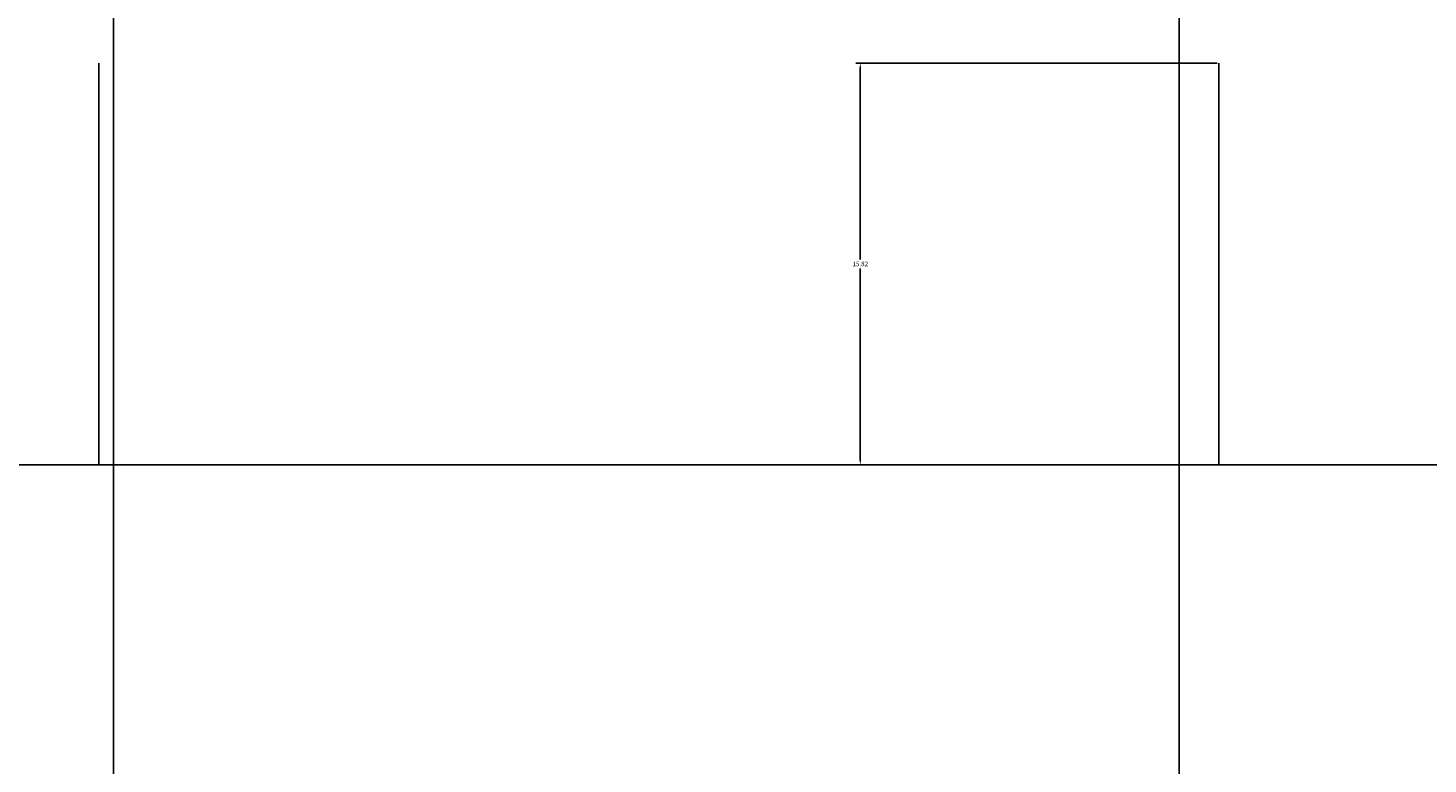
# Model space of a CAD drawing. Units: millimetres. Extents: x -8 to 285, y 5 to 221.
# Tile 21 of 30: x 186 to 241, y 103 to 132. Entities that reach past the tile are written whole.
import ezdxf

# ---------------------------------------------------------------- set-up
doc = ezdxf.new("R2010")
doc.units = ezdxf.units.MM
doc.layers.add('A-ANNO-DIMS', color=2, linetype='Continuous', lineweight=18)
doc.layers.add('E-POWR-AC-NEUT', color=3, linetype='Continuous', lineweight=25)
doc.styles.get("Standard").update_dxf_attribs({"font": 'arial.ttf'})
doc.dimstyles.get("Standard").update_dxf_attribs({"dimtxt": 0.18, "dimasz": 0.18, "dimexe": 0.18, "dimexo": 0.0625, "dimgap": 0.09, "dimtad": 0, "dimtih": 1, "dimtoh": 1, "dimdec": 4, "dimzin": 0, "dimdsep": 46, "dimtxsty": 'Standard', "dimcen": 0.09, "dimadec": 0, "dimazin": 0, "dimtfac": 1, "dimtdec": 4, "dimtofl": 0, "dimtmove": 0, "dimatfit": 3, "dimfxl": 1, "dimtolj": 1, "dimtzin": 0, "dimarcsym": 0})

# ---------------------------------------------------------------- blocks, each defined once
blk = doc.blocks.new('*D13')
at = {"layer": 'A-ANNO-DIMS', "color": 0, "lineweight": -2, "transparency": 16777216}
for p, q in [((145.21, 137.013), (145.21, 5.222)), ((189.039, 137.013), (189.039, 5.222)), ((145.39, 5.402), (166.727, 5.402)), ((188.859, 5.402), (167.522, 5.402))]:
    blk.add_line(p, q, dxfattribs=at)
at = {"layer": 'A-ANNO-DIMS', "color": 0, "transparency": 16777216}
for points in [[(145.39, 5.432), (145.39, 5.372), (145.21, 5.402)], [(188.859, 5.432), (188.859, 5.372), (189.039, 5.402)]]:
    blk.add_solid(points, dxfattribs=at)
at = {"layer": 'Defpoints', "color": 0, "transparency": 16777216}
for p in [(145.21, 137.075), (189.039, 137.075), (189.039, 5.402)]:
    blk.add_point(p, dxfattribs=at)
at = {"layer": 'A-ANNO-DIMS', "color": 0, "transparency": 16777216, "insert": (167.124, 5.402), "char_height": 0.18, "attachment_point": 5}
blk.add_mtext('\\A1;43.83', dxfattribs=at)
blk = doc.blocks.new('*D14')
at = {"layer": 'A-ANNO-DIMS', "color": 0, "lineweight": -2, "transparency": 16777216}
for p, q in [((189.039, 137.013), (189.039, 5.222)), ((230.967, 137.013), (230.967, 5.222)), ((189.219, 5.402), (209.606, 5.402)), ((230.787, 5.402), (210.4, 5.402))]:
    blk.add_line(p, q, dxfattribs=at)
at = {"layer": 'A-ANNO-DIMS', "color": 0, "transparency": 16777216}
for points in [[(189.219, 5.432), (189.219, 5.372), (189.039, 5.402)], [(230.787, 5.432), (230.787, 5.372), (230.967, 5.402)]]:
    blk.add_solid(points, dxfattribs=at)
at = {"layer": 'Defpoints', "color": 0, "transparency": 16777216}
for p in [(189.039, 137.075), (230.967, 137.075), (230.967, 5.402)]:
    blk.add_point(p, dxfattribs=at)
at = {"layer": 'A-ANNO-DIMS', "color": 0, "transparency": 16777216, "insert": (210.003, 5.402), "char_height": 0.18, "attachment_point": 5}
blk.add_mtext('\\A1;41.93', dxfattribs=at)
blk = doc.blocks.new('*D17')
at = {"layer": 'A-ANNO-DIMS', "color": 0, "lineweight": -2, "transparency": 16777216}
for p, q in [((232.455, 130.961), (218.237, 130.961)), ((218.417, 130.781), (218.417, 123.234)), ((218.417, 115.323), (218.417, 122.87)), ((232.455, 115.143), (218.237, 115.143))]:
    blk.add_line(p, q, dxfattribs=at)
at = {"layer": 'A-ANNO-DIMS', "color": 0, "transparency": 16777216}
for points in [[(218.387, 130.781), (218.447, 130.781), (218.417, 130.961)], [(218.387, 115.323), (218.447, 115.323), (218.417, 115.143)]]:
    blk.add_solid(points, dxfattribs=at)
at = {"layer": 'Defpoints', "color": 0, "transparency": 16777216}
for p in [(218.417, 130.961), (232.517, 130.961), (232.517, 115.143)]:
    blk.add_point(p, dxfattribs=at)
at = {"layer": 'A-ANNO-DIMS', "color": 0, "transparency": 16777216, "insert": (218.417, 123.052), "char_height": 0.18, "attachment_point": 5}
blk.add_mtext('\\A1;15.82', dxfattribs=at)

msp = doc.modelspace()

# ---------------------------------------------------------------- linework, layer by layer
at = {"layer": 'E-POWR-AC-NEUT'}
for p, q in [((188.4531, 130.9614), (188.4531, 115.1427)), ((232.5173, 130.9614), (232.5173, 115.1427))]:
    msp.add_line(p, q, dxfattribs=at)
msp.add_lwpolyline([(231.5468, 34.6512), (231.5468, 58.5666), (262.873, 58.5666), (262.873, 115.1427), (144.6762, 115.1427), (144.6762, 130.9614)], dxfattribs=at)

# ---------------------------------------------------------------- dimensions: what is measured, and where the dimension line sits
at = {"layer": 'A-ANNO-DIMS'}
for base, p1, p2, picture, middle in [((189.039, 5.402), (145.2095, 137.0752), (189.039, 137.0752), '*D13', (167.1243, 5.402)), ((230.9672, 5.402), (189.039, 137.0752), (230.9672, 137.0752), '*D14', (210.0031, 5.402))]:
    dim = msp.add_linear_dim(base=base, p1=p1, p2=p2, dimstyle='Standard', override={"dimdec": 2, "dimlfac": 1, "dimrnd": 0, "dimzin": 0, "dimdsep": 46, "dimlunit": 2}, dxfattribs=at)
    dim.commit()
    dim.dimension.update_dxf_attribs({"geometry": picture, "text_midpoint": middle})
dim = msp.add_linear_dim(base=(218.4173, 130.9614), p1=(232.5173, 115.1427), p2=(232.5173, 130.9614), angle=90, dimstyle='Standard', override={"dimdec": 2, "dimlfac": 1, "dimrnd": 0, "dimzin": 0, "dimdsep": 46, "dimlunit": 2}, dxfattribs=at)
dim.commit()
dim.dimension.update_dxf_attribs({"geometry": '*D17', "text_midpoint": (218.4173, 123.0521)})

doc.saveas('drawing.dxf')
